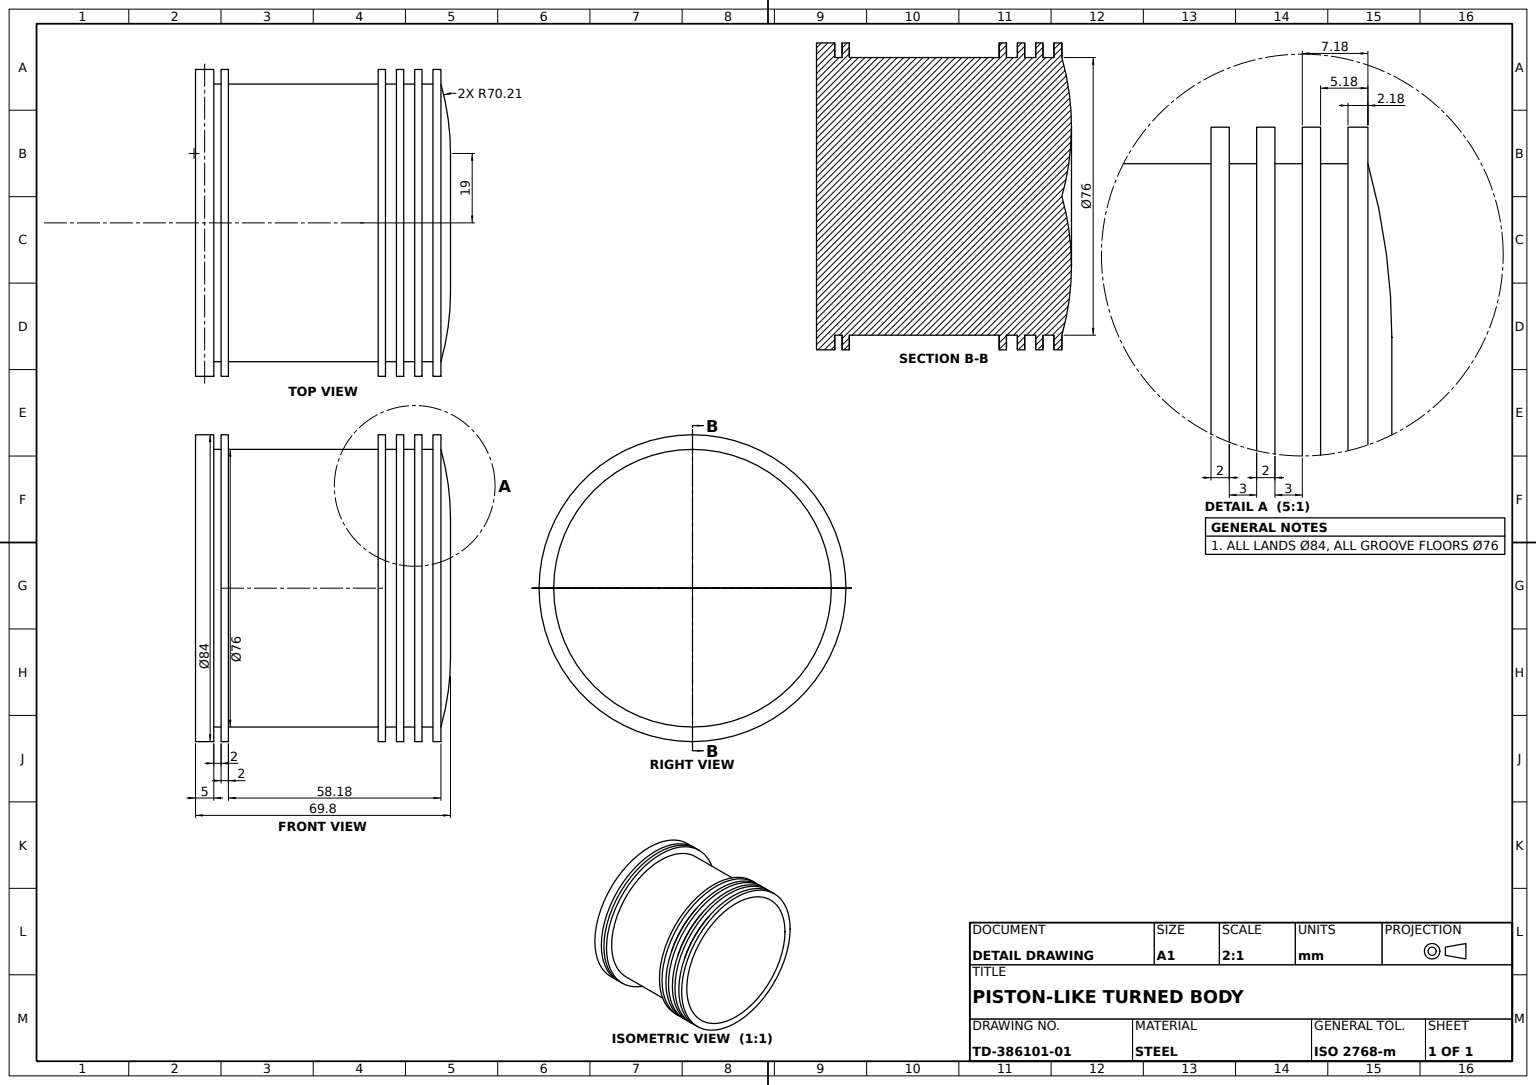
SolidWorks part; units mm, degrees
material "Plain Carbon Steel"
ref_plane "Front Plane" through (0, 0, 0) normal (0, 0, 1) x (1, 0, 0)
ref_plane "Top Plane" through (0, 0, 0) normal (0, 1, 0) x (1, 0, 0)
ref_plane "Right Plane" through (0, 0, 0) normal (1, 0, 0) x (0, 0, -1)
sketch "Piston Profile Sketch" plane through (0, 0, 0) normal (0, 0, 1) x (1, 0, 0)
  line L0 (0, 0) -> (37, 0)
  line L1 (37, 0) -> (42, 0)
  line L2 (42, 0) -> (42, 5)
  line L3 (42, 5) -> (38, 5)
  line L4 (38, 5) -> (38, 7)
  line L5 (42, 7) -> (38, 7)
  line L6 (42, 7) -> (42, 9)
  line L7 (42, 9) -> (38, 9)
  line L8 (0, 0) -> (0, 67.1822)
  line L9 (38, 62) -> (42, 62)
  line L10 (42, 62) -> (42, 60)
  line L11 (42, 60) -> (38, 60)
  line L12 (38, 60) -> (38, 57)
  line L13 (38, 57) -> (42, 57)
  line L14 (42, 57) -> (42, 55)
  line L15 (42, 55) -> (38, 55)
  line L16 (38, 55) -> (38, 52)
  line L17 (38, 52) -> (42, 52)
  line L18 (42, 52) -> (42, 50)
  line L19 (42, 50) -> (38, 50)
  line L20 (38, 65) -> (38, 62)
  line L21 (38, 67.1822) -> (42, 67.1822)
  line L22 (42, 67.1822) -> (42, 65)
  line L23 (42, 65) -> (38, 65)
  line L24 (0, 0) -> (0, 67.1822) construction
  line L26 (38, 50) -> (38, 9)
  arc A0 (0, 67.1822) -> (38, 67.1822) centre (19, -0.4076) cw
  point P3 (0, 0)
  dimension "D4" = 19
  dimension "D2" = 70.2095
  dimension "D1" = 5
  dimension "D3" = 5
  dimension "D5" = 37
  dimension "D6" = 2.1822
  dimension "D7" = 5.1822
  dimension "D8" = 7.1822
  dimension "D9" = 58.1822
revolve "Piston Body Revolve" add sketch "Piston Profile Sketch" angle 360 about L24
